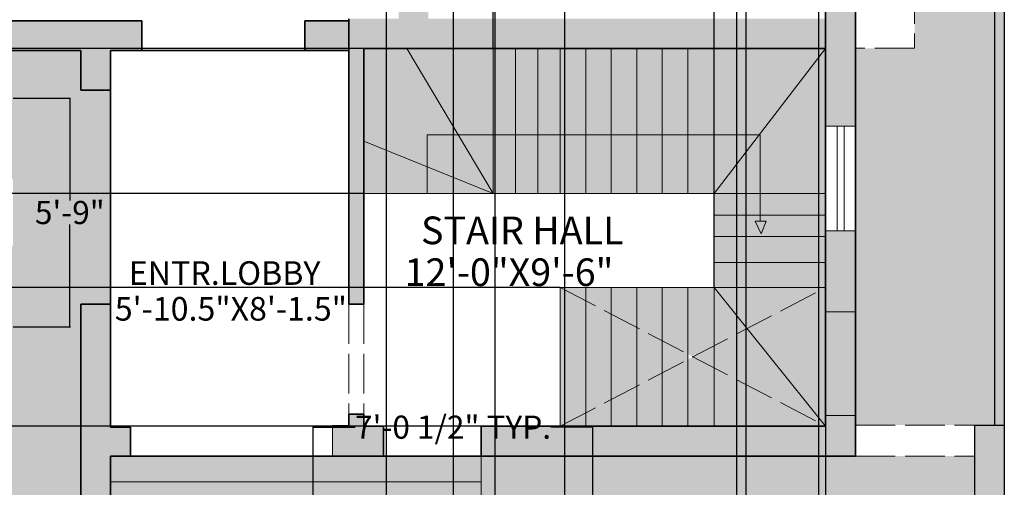
# Model space of a CAD drawing. Units: inches. Extents: x 1884 to 2398, y 474 to 1488.
# Tile 33 of 39: x 2099 to 2397, y 761 to 902. Entities that reach past the tile are written whole.
import ezdxf

# ---------------------------------------------------------------- set-up
doc = ezdxf.new("R2010")
doc.units = ezdxf.units.IN
doc.header["$MEASUREMENT"] = 0
doc.linetypes.add('ACAD_ISO02W100', pattern=[15, 12, -3])
for name, color, linetype, lineweight in [('A-ANNO-DIMS', 2, 'Continuous', 18), ('A-ANNO-SYMB', 7, 'Continuous', 18), ('A-AREA-IDEN', 7, 'Continuous', 18), ('A-FLOR-OVHD', 8, 'ACAD_ISO02W100', 18), ('A-FLOR-PATT', 254, 'Continuous', 13), ('A-FLOR-STRS', 7, 'Continuous', 20), ('A-FLOR-STRS-HIDN', 8, 'ACAD_ISO02W100', 18), ('A-WALL-PATT', 250, 'Continuous', 13), ('C-PROP', 7, 'Continuous', 30), ('walls', 7, 'Continuous', 35), ('windows', 4, 'Continuous', 18)]:
    doc.layers.add(name, color=color, linetype=linetype, lineweight=lineweight)
for name, color, linetype, lineweight, true_color in [('A-FLOR-STRS-PATT', 251, 'Continuous', 13, 0x636466), ('A-GLAZ-PATT', 7, 'Continuous', 13, 0xf5f5f5), ('L-PVMT-PATT', 9, 'Continuous', 13, 0xc7c8ca)]:
    doc.layers.add(name, color=color, linetype=linetype, lineweight=lineweight, true_color=true_color)
doc.styles.get("Standard").update_dxf_attribs({"font": 'arial.ttf'})
doc.dimstyles.get("Standard").update_dxf_attribs({"dimtxt": 7, "dimasz": 0.18, "dimexe": 0.18, "dimexo": 0.0625, "dimgap": 0.09, "dimtad": 0, "dimtih": 1, "dimtoh": 1, "dimzin": 0, "dimdsep": 46, "dimlunit": 3, "dimtxsty": 'Standard', "dimcen": 0.09, "dimadec": 0, "dimazin": 0, "dimtfac": 1, "dimtofl": 0, "dimtmove": 0, "dimatfit": 3, "dimfxl": 1, "dimtolj": 1, "dimtzin": 0, "dimarcsym": 0})

# ---------------------------------------------------------------- blocks, each defined once
blk = doc.blocks.new('*D24')
at = {"layer": 'A-ANNO-DIMS', "color": 0, "lineweight": -2, "transparency": 16777216}
for p, q in [((2187.71, 752.87), (2187.71, 778.86)), ((2187.89, 778.68), (2200.43, 778.68)), ((2272.06, 778.68), (2259.53, 778.68)), ((2272.24, 752.87), (2272.24, 778.86))]:
    blk.add_line(p, q, dxfattribs=at)
at = {"layer": 'A-ANNO-DIMS', "color": 0, "lineweight": 100, "transparency": 16777216}
for points in [[(2187.89, 778.71), (2187.89, 778.65), (2187.71, 778.68)], [(2272.06, 778.71), (2272.06, 778.65), (2272.24, 778.68)]]:
    blk.add_solid(points, dxfattribs=at)
at = {"layer": 'Defpoints', "color": 0, "lineweight": 100, "transparency": 16777216}
for p in [(2272.24, 778.68), (2187.71, 752.81), (2272.24, 752.81)]:
    blk.add_point(p, dxfattribs=at)
at = {"layer": 'A-ANNO-DIMS', "color": 0, "transparency": 16777216, "insert": (2229.98, 778.68), "char_height": 7, "attachment_point": 5}
blk.add_mtext('\\A1;7\'-0 1/2" TYP.', dxfattribs=at)
blk = doc.blocks.new('*D36')
at = {"layer": 'A-ANNO-DIMS', "color": 0, "lineweight": -2, "transparency": 16777216}
for p, q in [((2097.11, 878.02), (2114.37, 878.02)), ((2114.19, 877.84), (2114.19, 847.14)), ((2114.19, 809.11), (2114.19, 839.81)), ((2097.11, 808.93), (2114.37, 808.93))]:
    blk.add_line(p, q, dxfattribs=at)
at = {"layer": 'A-ANNO-DIMS', "color": 0, "lineweight": 100, "transparency": 16777216}
for points in [[(2114.16, 877.84), (2114.22, 877.84), (2114.19, 878.02)], [(2114.16, 809.11), (2114.22, 809.11), (2114.19, 808.93)]]:
    blk.add_solid(points, dxfattribs=at)
at = {"layer": 'Defpoints', "color": 0, "lineweight": 100, "transparency": 16777216}
for p in [(2097.04, 878.02), (2097.04, 808.93), (2114.19, 808.93)]:
    blk.add_point(p, dxfattribs=at)
at = {"layer": 'A-ANNO-DIMS', "color": 0, "transparency": 16777216, "insert": (2114.19, 843.48), "char_height": 7, "attachment_point": 5}
blk.add_mtext('\\A1;5\'-9"', dxfattribs=at)
blk = doc.blocks.new('*D44')
at = {"layer": 'A-ANNO-DIMS', "color": 0, "lineweight": -2, "transparency": 16777216}
for p, q in [((2209.76, 1247.82), (2209.76, 484)), ((2230.03, 1247.82), (2230.03, 484)), ((2209.94, 484.18), (2229.85, 484.18)), ((2230.03, 484.18), (2230.21, 484.18))]:
    blk.add_line(p, q, dxfattribs=at)
at = {"layer": 'A-ANNO-DIMS', "color": 0, "lineweight": 100, "transparency": 16777216}
for points in [[(2209.94, 484.21), (2209.94, 484.15), (2209.76, 484.18)], [(2229.85, 484.21), (2229.85, 484.15), (2230.03, 484.18)]]:
    blk.add_solid(points, dxfattribs=at)
at = {"layer": 'Defpoints', "color": 0, "lineweight": 100, "transparency": 16777216}
for p in [(2209.76, 1247.88), (2230.03, 1247.88), (2230.03, 484.18)]:
    blk.add_point(p, dxfattribs=at)
at = {"layer": 'A-ANNO-DIMS', "color": 0, "transparency": 16777216, "insert": (2247.43, 484.18), "char_height": 7, "attachment_point": 5}
blk.add_mtext('\\A1;1\'-8 1/2"', dxfattribs=at)
blk = doc.blocks.new('*D45')
at = {"layer": 'A-ANNO-DIMS', "color": 0, "lineweight": -2, "transparency": 16777216}
for p, q in [((2242.62, 1322.82), (2242.62, 484)), ((2263.62, 1322.82), (2263.62, 484)), ((2242.8, 484.18), (2244.05, 484.18)), ((2263.44, 484.18), (2262.18, 484.18))]:
    blk.add_line(p, q, dxfattribs=at)
at = {"layer": 'A-ANNO-DIMS', "color": 0, "lineweight": 100, "transparency": 16777216}
for points in [[(2242.8, 484.21), (2242.8, 484.15), (2242.62, 484.18)], [(2263.44, 484.21), (2263.44, 484.15), (2263.62, 484.18)]]:
    blk.add_solid(points, dxfattribs=at)
at = {"layer": 'Defpoints', "color": 0, "lineweight": 100, "transparency": 16777216}
for p in [(2242.62, 1322.88), (2263.62, 1322.88), (2263.62, 484.18)]:
    blk.add_point(p, dxfattribs=at)
at = {"layer": 'A-ANNO-DIMS', "color": 0, "transparency": 16777216, "insert": (2253.12, 484.18), "char_height": 7, "attachment_point": 5}
blk.add_mtext('\\A1;1\'-9"', dxfattribs=at)
blk = doc.blocks.new('*D47')
at = {"layer": 'A-ANNO-DIMS', "color": 0, "lineweight": -2, "transparency": 16777216}
for p, q in [((2315.59, 959.7), (2315.59, 484)), ((2342.53, 959.7), (2342.53, 484)), ((2315.77, 484.18), (2319.61, 484.18)), ((2342.35, 484.18), (2338.51, 484.18))]:
    blk.add_line(p, q, dxfattribs=at)
at = {"layer": 'A-ANNO-DIMS', "color": 0, "lineweight": 100, "transparency": 16777216}
for points in [[(2315.77, 484.21), (2315.77, 484.15), (2315.59, 484.18)], [(2342.35, 484.21), (2342.35, 484.15), (2342.53, 484.18)]]:
    blk.add_solid(points, dxfattribs=at)
at = {"layer": 'Defpoints', "color": 0, "lineweight": 100, "transparency": 16777216}
for p in [(2315.59, 959.77), (2342.53, 959.77), (2342.53, 484.18)]:
    blk.add_point(p, dxfattribs=at)
at = {"layer": 'A-ANNO-DIMS', "color": 0, "transparency": 16777216, "insert": (2329.06, 484.18), "char_height": 7, "attachment_point": 5}
blk.add_mtext('\\A1;2\'-3"', dxfattribs=at)
blk = doc.blocks.new('*D49')
at = {"layer": 'A-ANNO-DIMS', "color": 0, "lineweight": -2, "transparency": 16777216}
for p, q in [((2318.41, 987.72), (2318.41, 484)), ((2340.41, 987.72), (2340.41, 484)), ((2318.59, 484.18), (2340.23, 484.18)), ((2340.41, 484.18), (2340.59, 484.18))]:
    blk.add_line(p, q, dxfattribs=at)
at = {"layer": 'A-ANNO-DIMS', "color": 0, "lineweight": 100, "transparency": 16777216}
for points in [[(2318.59, 484.21), (2318.59, 484.15), (2318.41, 484.18)], [(2340.23, 484.21), (2340.23, 484.15), (2340.41, 484.18)]]:
    blk.add_solid(points, dxfattribs=at)
at = {"layer": 'Defpoints', "color": 0, "lineweight": 100, "transparency": 16777216}
for p in [(2318.41, 987.78), (2340.41, 987.78), (2340.41, 484.18)]:
    blk.add_point(p, dxfattribs=at)
at = {"layer": 'A-ANNO-DIMS', "color": 0, "transparency": 16777216, "insert": (2352.37, 484.18), "char_height": 7, "attachment_point": 5}
blk.add_mtext('\\A1;1\'-10"', dxfattribs=at)
blk = doc.blocks.new('*D51')
at = {"layer": 'A-ANNO-DIMS', "color": 0, "lineweight": -2, "transparency": 16777216}
for p, q in [((2202.97, 892.97), (1902.43, 892.97)), ((1902.61, 892.79), (1902.61, 874.82)), ((1902.61, 849.42), (1902.61, 867.39)), ((2202.97, 849.24), (1902.43, 849.24))]:
    blk.add_line(p, q, dxfattribs=at)
at = {"layer": 'A-ANNO-DIMS', "color": 0, "lineweight": 100, "transparency": 16777216}
for points in [[(1902.58, 892.79), (1902.64, 892.79), (1902.61, 892.97)], [(1902.58, 849.42), (1902.64, 849.42), (1902.61, 849.24)]]:
    blk.add_solid(points, dxfattribs=at)
at = {"layer": 'Defpoints', "color": 0, "lineweight": 100, "transparency": 16777216}
for p in [(1902.61, 892.97), (2203.03, 892.97), (2203.03, 849.24)]:
    blk.add_point(p, dxfattribs=at)
at = {"layer": 'A-ANNO-DIMS', "color": 0, "transparency": 16777216, "insert": (1902.61, 871.1), "char_height": 7, "attachment_point": 5}
blk.add_mtext('\\A1;3\'-7 1/2"', dxfattribs=at)
blk = doc.blocks.new('*D52')
at = {"layer": 'A-ANNO-DIMS', "color": 0, "lineweight": -2, "transparency": 16777216}
for p, q in [((2308.85, 820.89), (2308.85, 1477.76)), ((2309.03, 1477.58), (2342.35, 1477.58)), ((2342.53, 820.89), (2342.53, 1477.76)), ((2342.53, 1477.58), (2342.71, 1477.58))]:
    blk.add_line(p, q, dxfattribs=at)
at = {"layer": 'A-ANNO-DIMS', "color": 0, "lineweight": 100, "transparency": 16777216}
for points in [[(2309.03, 1477.61), (2309.03, 1477.55), (2308.85, 1477.58)], [(2342.35, 1477.61), (2342.35, 1477.55), (2342.53, 1477.58)]]:
    blk.add_solid(points, dxfattribs=at)
at = {"layer": 'Defpoints', "color": 0, "lineweight": 100, "transparency": 16777216}
for p in [(2342.53, 1477.58), (2308.85, 820.83), (2342.53, 820.83)]:
    blk.add_point(p, dxfattribs=at)
at = {"layer": 'A-ANNO-DIMS', "color": 0, "transparency": 16777216, "insert": (2360.32, 1477.58), "char_height": 7, "attachment_point": 5}
blk.add_mtext('\\A1;2\'-9 1/2"', dxfattribs=at)
blk = doc.blocks.new('*D53')
at = {"layer": 'A-ANNO-DIMS', "color": 0, "lineweight": -2, "transparency": 16777216}
for p, q in [((2262.32, 820.83), (1902.43, 820.83)), ((1902.61, 820.65), (1902.61, 803.56)), ((1902.61, 779.15), (1902.61, 796.23)), ((2262.32, 778.97), (1902.43, 778.97))]:
    blk.add_line(p, q, dxfattribs=at)
at = {"layer": 'A-ANNO-DIMS', "color": 0, "lineweight": 100, "transparency": 16777216}
for points in [[(1902.58, 820.65), (1902.64, 820.65), (1902.61, 820.83)], [(1902.58, 779.15), (1902.64, 779.15), (1902.61, 778.97)]]:
    blk.add_solid(points, dxfattribs=at)
at = {"layer": 'Defpoints', "color": 0, "lineweight": 100, "transparency": 16777216}
for p in [(1902.61, 820.83), (2262.38, 820.83), (2262.38, 778.97)]:
    blk.add_point(p, dxfattribs=at)
at = {"layer": 'A-ANNO-DIMS', "color": 0, "transparency": 16777216, "insert": (1902.61, 799.9), "char_height": 7, "attachment_point": 5}
blk.add_mtext('\\A1;3\'-6"', dxfattribs=at)
blk = doc.blocks.new('*D54')
at = {"layer": 'A-ANNO-DIMS', "color": 0, "lineweight": -2, "transparency": 16777216}
for p, q in [((2242.06, 893.03), (2242.06, 1477.76)), ((2242.24, 1477.58), (2266.06, 1477.58)), ((2308.67, 1477.58), (2284.85, 1477.58)), ((2308.85, 893.03), (2308.85, 1477.76))]:
    blk.add_line(p, q, dxfattribs=at)
at = {"layer": 'A-ANNO-DIMS', "color": 0, "lineweight": 100, "transparency": 16777216}
for points in [[(2242.24, 1477.61), (2242.24, 1477.55), (2242.06, 1477.58)], [(2308.67, 1477.61), (2308.67, 1477.55), (2308.85, 1477.58)]]:
    blk.add_solid(points, dxfattribs=at)
at = {"layer": 'Defpoints', "color": 0, "lineweight": 100, "transparency": 16777216}
for p in [(2308.85, 1477.58), (2242.06, 892.97), (2308.85, 892.97)]:
    blk.add_point(p, dxfattribs=at)
at = {"layer": 'A-ANNO-DIMS', "color": 0, "transparency": 16777216, "insert": (2275.45, 1477.58), "char_height": 7, "attachment_point": 5}
blk.add_mtext('\\A1;5\'-7"', dxfattribs=at)

msp = doc.modelspace()

# ---------------------------------------------------------------- hatches: boundary and pattern name
at = {"layer": 'A-ANNO-SYMB'}
h = msp.add_hatch(color=256, dxfattribs=at)
h.dxf.hatch_style = 1
h.paths.add_polyline_path([(2324.539, 840.913), (2323.026, 840.913), (2321.211, 840.913), (2323.026, 837.06)])
at = {"layer": 'A-FLOR-PATT'}
h = msp.add_hatch(color=256, dxfattribs=at)
h.dxf.hatch_style = 1
h.paths.add_polyline_path([(2117.529, 815.801), (2126.529, 815.801), (2126.529, 880.382), (2117.529, 880.382), (2117.529, 892.385), (1961.529, 892.385), (1961.529, 756.915), (1964.529, 756.915), (1964.529, 759.915), (1995.529, 759.915), (1995.529, 753.915), (1972.862, 753.915), (1967.529, 756.915), (1967.529, 654.915), (1972.862, 657.915), (1995.529, 657.915), (1995.529, 651.915), (1964.529, 651.915), (1964.529, 654.915), (1961.529, 654.915), (1961.529, 640.385), (2117.529, 640.385), (2117.529, 646.578), (2126.529, 646.578), (2126.529, 676.183), (2117.529, 676.183)])
h.paths.add_polyline_path([(2012.246, 808.929), (2012.05, 810.185), (2032.542, 810.185), (2032.346, 808.929)], flags=16)
h.paths.add_polyline_path([(2010.381, 820.864), (1994.658, 820.864), (1994.658, 831.561), (1984.608, 833.132), (1984.608, 853.821), (1994.658, 855.391), (1994.658, 866.089), (2010.381, 866.089), (2011.951, 876.139), (2032.64, 876.139), (2034.211, 866.089), (2045.556, 866.089), (2047.127, 876.139), (2067.816, 876.139), (2069.386, 866.089), (2085.109, 866.089), (2085.109, 855.391), (2095.159, 853.821), (2095.159, 833.132), (2085.109, 831.561), (2085.109, 820.864), (2069.386, 820.864), (2067.816, 810.814), (2047.127, 810.814), (2045.556, 820.864), (2034.211, 820.864), (2032.64, 810.814), (2011.951, 810.814)], flags=16)
h.paths.add_polyline_path([(1982.724, 833.426), (1982.724, 853.526), (1983.98, 853.723), (1983.98, 833.23)], flags=16)
h.paths.add_polyline_path([(1994.529, 753.54), (1994.529, 658.29), (1973.529, 658.29), (1973.529, 753.54)], flags=16)
h.paths.add_polyline_path([(2084.486, 843.527), (2084.592, 843.502), (2084.681, 843.487), (2084.813, 843.477), (2084.913, 843.477), (2084.669, 843.482), (2084.336, 843.565), (2084.116, 843.617), (2083.8, 843.686), (2083.105, 843.827), (2082.836, 843.874), (2083.604, 843.729), (2084.206, 843.597)], flags=0)
h.paths.add_polyline_path([(2047.421, 808.929), (2047.225, 810.185), (2067.718, 810.185), (2067.521, 808.929)], flags=16)
h.paths.add_polyline_path([(2066.01, 849.505), (2066.429, 849.687), (2066.798, 849.882), (2067.129, 850.085), (2067.43, 850.293), (2067.711, 850.502), (2068.176, 850.856), (2068.689, 851.205), (2069.305, 851.531), (2070.015, 851.784), (2070.844, 851.944), (2071.081, 851.956), (2070.629, 851.902), (2070.212, 851.822), (2069.827, 851.717), (2069.471, 851.59), (2069.139, 851.443), (2068.828, 851.279), (2068.534, 851.1), (2068.254, 850.909), (2067.983, 850.709), (2067.502, 850.343), (2066.951, 849.962), (2066.224, 849.579)], flags=0)
h.paths.add_polyline_path([(2059.423, 853.221), (2059.827, 853.278), (2060.171, 853.358), (2060.465, 853.463), (2060.714, 853.589), (2060.926, 853.736), (2061.107, 853.902), (2061.258, 854.086), (2061.377, 854.284), (2061.462, 854.495), (2061.514, 854.715), (2061.53, 854.943), (2061.508, 855.176), (2061.449, 855.411), (2061.352, 855.646), (2061.224, 855.882), (2061.07, 856.117), (2060.9, 856.353), (2060.719, 856.588), (2060.406, 856.993), (2060.103, 857.424), (2059.858, 857.888), (2059.691, 858.467), (2059.836, 859.091), (2060.305, 859.532), (2060.844, 859.798), (2061.513, 859.935), (2062.253, 859.905), (2062.483, 859.849), (2062.078, 859.912), (2061.695, 859.928), (2061.336, 859.899), (2061.005, 859.831), (2060.703, 859.729), (2060.437, 859.597), (2060.208, 859.441), (2060.021, 859.265), (2059.879, 859.075), (2059.785, 858.874), (2059.737, 858.664), (2059.73, 858.447), (2059.761, 858.224), (2059.827, 857.996), (2059.923, 857.765), (2060.047, 857.53), (2060.193, 857.295), (2060.359, 857.06), (2060.537, 856.824), (2060.867, 856.399), (2061.171, 855.978), (2061.422, 855.518), (2061.567, 854.943), (2061.41, 854.272), (2060.947, 853.707), (2060.335, 853.397), (2059.649, 853.236)], flags=0)
h.paths.add_polyline_path([(2050.778, 859.745), (2051.07, 859.87), (2051.295, 860.017), (2051.467, 860.183), (2051.594, 860.365), (2051.679, 860.56), (2051.726, 860.763), (2051.739, 860.971), (2051.722, 861.18), (2051.677, 861.387), (2051.609, 861.587), (2051.521, 861.779), (2051.421, 861.962), (2051.312, 862.138), (2051.203, 862.307), (2050.966, 862.68), (2050.793, 863.193), (2051.021, 863.699), (2051.483, 864.018), (2052.09, 864.138), (2052.773, 864.157), (2053.007, 864.142), (2052.603, 864.152), (2052.258, 864.142), (2051.965, 864.113), (2051.716, 864.064), (2051.504, 863.995), (2051.322, 863.907), (2051.17, 863.802), (2051.048, 863.682), (2050.954, 863.55), (2050.891, 863.408), (2050.856, 863.259), (2050.851, 863.105), (2050.876, 862.948), (2050.929, 862.791), (2051.005, 862.633), (2051.098, 862.472), (2051.203, 862.307), (2051.312, 862.138), (2051.556, 861.742), (2051.751, 861.167), (2051.712, 860.535), (2051.398, 860.085), (2050.949, 859.79)], flags=0)
h.paths.add_polyline_path([(2022.768, 719.264), (2050.461, 719.264), (2050.461, 717.226), (2052.426, 717.226), (2052.426, 715.033), (2050.461, 715.033), (2050.461, 703.738), (2022.768, 703.738)], flags=16)
h.paths.add_polyline_path([(2012.246, 878.023), (2032.346, 878.023), (2032.542, 876.767), (2012.05, 876.767)], flags=16)
h.paths.add_polyline_path([(2035.324, 713.103), (2035.342, 713.294), (2035.192, 713.202)], flags=0)
h.paths.add_polyline_path([(2036.484, 711.63), (2036.583, 711.849), (2036.39, 711.898)], flags=0)
h.paths.add_polyline_path([(2036.074, 712.744), (2035.993, 712.481), (2035.724, 712.516), (2035.794, 712.726)], flags=0)
h.paths.add_polyline_path([(2035.846, 710.909), (2035.753, 710.958), (2035.702, 710.88)], flags=0)
h.paths.add_polyline_path([(2037.818, 712.019), (2037.948, 712.06), (2037.987, 712.161), (2037.815, 712.02)], flags=0)
h.paths.add_polyline_path([(2038.451, 709.517), (2038.464, 709.428), (2038.586, 709.442)], flags=0)
h.paths.add_polyline_path([(2037.805, 709.806), (2037.818, 709.807), (2037.804, 709.823)], flags=0)
h.paths.add_polyline_path([(2036.7, 711.245), (2036.698, 711.236), (2036.813, 711.211)], flags=0)
h.paths.add_polyline_path([(2035.928, 708.897), (2035.668, 708.871), (2035.706, 708.667)], flags=0)
h.paths.add_polyline_path([(2036.414, 710.976), (2035.932, 709.859), (2036.792, 710.484), (2036.5, 710.934)], flags=0)
h.paths.add_polyline_path([(2038.298, 712.115), (2038.499, 712.058), (2038.612, 712.269), (2038.39, 712.332)], flags=0)
h.paths.add_polyline_path([(2047.421, 878.023), (2067.521, 878.023), (2067.718, 876.767), (2047.225, 876.767)], flags=16)
h.paths.add_polyline_path([(2049.647, 705.093, -1), (2048.845, 705.093, -1)], flags=0)
h.paths.add_polyline_path([(2095.787, 853.723), (2097.043, 853.526), (2097.043, 833.426), (2095.787, 833.23)], flags=16)
h.paths.add_polyline_path([(2110.739, 745.339), (2111.75, 745.339, -0.0640419), (2113.267, 742.92), (2113.267, 732.192), (2113.526, 732.192, -0.4142136), (2114.278, 731.439), (2114.278, 716.764, -0.4142136), (2113.526, 716.011), (2113.267, 716.011), (2113.267, 705.284, -0.0640419), (2111.75, 702.864), (2110.739, 702.864), (2110.739, 716.011), (2109.469, 716.011, -0.4142136), (2108.716, 716.764), (2108.716, 731.439, -0.4142136), (2109.469, 732.192), (2110.739, 732.192)], flags=16)
h.paths.add_polyline_path([(1998.045, 668.909), (2002.449, 668.909), (2002.449, 652.273), (2002.724, 652.763), (2002.724, 668.175), (2019.972, 668.175), (2019.972, 652.763), (2020.247, 652.273), (2020.247, 668.909), (2024.651, 668.909), (2029.055, 668.909), (2029.055, 652.273), (2029.33, 652.763), (2029.33, 668.175), (2046.578, 668.175), (2046.578, 652.763), (2046.853, 652.273), (2046.853, 668.909), (2051.257, 668.909), (2051.257, 646.157), (2049.055, 646.157), (2049.055, 643.955), (2026.853, 643.955), (2026.853, 646.157), (2024.651, 646.157), (2022.449, 646.157), (2022.449, 643.955), (2000.247, 643.955), (2000.247, 646.157), (1998.045, 646.157)], flags=16)
h.paths.add_polyline_path([(2342.529, 1247.885), (2265.892, 1247.885), (2230.029, 1247.885), (2209.755, 1247.885), (2168.6, 1247.885), (2168.6, 1104.929), (2158.029, 1104.929), (2158.029, 1079.411), (2168.6, 1079.411), (2168.6, 1062.466), (2342.529, 1062.466), (2342.529, 1093.809)])
h.paths.add_polyline_path([(2215.03, 1153.876), (2215.03, 1164.739), (2187.559, 1164.739), (2187.442, 1152.641), (2173.568, 1152.641), (2173.684, 1164.739), (2173.684, 1218.739), (2173.801, 1230.837), (2187.675, 1230.837), (2187.559, 1218.739), (2215.03, 1218.739), (2215.03, 1225.879), (2245.053, 1225.879), (2245.053, 1153.876)], flags=16)
h.paths.add_polyline_path([(2192.147, 1164.797), (2184.963, 1174.54), (2184.915, 1174.54), (2176.755, 1174.54), (2176.755, 1190.363), (2184.915, 1190.363), (2184.915, 1196.819), (2176.755, 1196.819), (2176.755, 1212.641), (2184.915, 1212.641), (2184.915, 1174.606), (2184.963, 1174.54), (2192.147, 1174.54)], flags=0)
h.paths.add_polyline_path([(2184.971, 1158.364, -1), (2176.039, 1158.364, -1)], flags=0)
h.paths.add_polyline_path([(2335.555, 1161.985), (2335.555, 1175.132), (2334.285, 1175.132, -0.4142136), (2333.533, 1175.885), (2333.533, 1190.56, -0.4142136), (2334.285, 1191.313), (2335.555, 1191.313), (2335.555, 1204.46), (2336.567, 1204.46, -0.0640419), (2338.083, 1202.04), (2338.083, 1191.313), (2338.342, 1191.313, -0.4142136), (2339.095, 1190.56), (2339.095, 1175.885, -0.4142136), (2338.342, 1175.132), (2338.083, 1175.132), (2338.083, 1164.405, -0.0640419), (2336.567, 1161.985)], flags=16)
h.paths.add_polyline_path([(2176.155, 1224.462, -1), (2185.087, 1224.462, -1)], flags=0)
h.paths.add_polyline_path([(2158.029, 1276.197), (2158.029, 1322.885), (2148.233, 1322.885), (2092.029, 1322.885), (1961.529, 1322.885), (1961.529, 1166.885), (2116.005, 1166.885), (2116.005, 1157.885), (2152.638, 1157.885), (2152.638, 1166.885), (2158.029, 1166.885)])
h.paths.add_polyline_path([(2006.352, 1204.245), (2006.352, 1215.108), (1978.881, 1215.108), (1978.764, 1203.01), (1964.89, 1203.01), (1965.006, 1215.108), (1965.006, 1269.108), (1965.123, 1281.207), (1978.997, 1281.207), (1978.881, 1269.108), (2006.352, 1269.108), (2006.352, 1276.248), (2036.375, 1276.248), (2036.375, 1204.245)], flags=16)
h.paths.add_polyline_path([(1983.469, 1215.166), (1976.285, 1224.909), (1976.237, 1224.909), (1968.077, 1224.909), (1968.077, 1240.732), (1976.237, 1240.732), (1976.237, 1247.188), (1968.077, 1247.188), (1968.077, 1263.011), (1976.237, 1263.011), (1976.237, 1224.975), (1976.285, 1224.909), (1983.469, 1224.909)], flags=0)
h.paths.add_polyline_path([(1976.293, 1208.733, -1), (1967.361, 1208.733, -1)], flags=0)
h.paths.add_polyline_path([(1967.477, 1274.832, -1), (1976.41, 1274.832, -1)], flags=0)
h.paths.add_polyline_path([(2152.587, 1223.485), (2152.587, 1236.632), (2151.317, 1236.632, -0.4142136), (2150.564, 1237.385), (2150.564, 1252.06, -0.4142136), (2151.317, 1252.813), (2152.587, 1252.813), (2152.587, 1265.959), (2153.598, 1265.959, -0.0640419), (2155.115, 1263.54), (2155.115, 1252.813), (2155.374, 1252.813, -0.4142136), (2156.126, 1252.06), (2156.126, 1237.385, -0.4142136), (2155.374, 1236.632), (2155.115, 1236.632), (2155.115, 1225.904, -0.0640419), (2153.598, 1223.485)], flags=16)
h.paths.add_polyline_path([(2250.676, 1161.101), (2322.077, 1161.101), (2322.077, 1173.886), (2250.676, 1173.886)], flags=24)
h.paths.add_polyline_path([(2255.61, 1173.712), (2320.136, 1173.712), (2320.136, 1186.659), (2255.61, 1186.659)], flags=24)
h.paths.add_polyline_path([(2053.687, 1230.837), (2125.089, 1230.837), (2125.089, 1243.622), (2053.687, 1243.622)], flags=24)
h.paths.add_polyline_path([(2058.622, 1243.448), (2123.147, 1243.448), (2123.147, 1256.395), (2058.622, 1256.395)], flags=24)
at = {"layer": 'A-FLOR-STRS-PATT'}
h = msp.add_hatch(color=256, dxfattribs=at)
h.dxf.hatch_style = 1
h.paths.add_polyline_path([(2215.996, 892.966), (2203.029, 892.966), (2203.029, 865.024), (2222.194, 857.274), (2222.194, 866.959), (2231.498, 866.959)])
h.paths.add_polyline_path([(2242.059, 892.966), (2215.996, 892.966), (2231.498, 866.959), (2242.059, 866.959)])
h.paths.add_polyline_path([(2231.498, 866.959), (2222.194, 866.959), (2222.194, 857.274), (2242.059, 849.241)])
h.paths.add_polyline_path([(2242.059, 866.959), (2231.498, 866.959), (2242.059, 849.241)], flags=17)
h.paths.add_polyline_path([(2222.194, 857.274), (2203.029, 865.024), (2203.029, 849.241), (2222.194, 849.241)])
h.paths.add_polyline_path([(2222.194, 857.274), (2222.194, 849.241), (2242.059, 849.241)], flags=17)
h.paths.add_polyline_path([(2248.833, 866.959), (2242.059, 866.959), (2242.059, 849.241), (2248.833, 849.241)])
h.paths.add_polyline_path([(2248.833, 892.966), (2242.059, 892.966), (2242.059, 866.959), (2248.833, 866.959)])
h.paths.add_polyline_path([(2255.607, 866.959), (2248.833, 866.959), (2248.833, 849.241), (2255.607, 849.241)])
h.paths.add_polyline_path([(2255.607, 892.966), (2248.833, 892.966), (2248.833, 866.959), (2255.607, 866.959)])
h.paths.add_polyline_path([(2262.382, 866.959), (2255.607, 866.959), (2255.607, 849.241), (2262.382, 849.241)])
h.paths.add_polyline_path([(2262.382, 892.966), (2255.607, 892.966), (2255.607, 866.959), (2262.382, 866.959)])
h.paths.add_polyline_path([(2270.083, 866.959), (2262.382, 866.959), (2262.382, 849.241), (2270.083, 849.241)])
h.paths.add_polyline_path([(2270.083, 892.966), (2262.382, 892.966), (2262.382, 866.959), (2270.083, 866.959)])
h.paths.add_polyline_path([(2277.785, 866.959), (2270.083, 866.959), (2270.083, 849.241), (2277.785, 849.241)])
h.paths.add_polyline_path([(2277.785, 892.966), (2270.083, 892.966), (2270.083, 866.959), (2277.785, 866.959)])
h.paths.add_polyline_path([(2285.487, 866.959), (2277.785, 866.959), (2277.785, 849.241), (2285.487, 849.241)])
h.paths.add_polyline_path([(2285.487, 892.966), (2277.785, 892.966), (2277.785, 866.959), (2285.487, 866.959)])
h.paths.add_polyline_path([(2293.189, 866.959), (2285.487, 866.959), (2285.487, 849.241), (2293.189, 849.241)])
h.paths.add_polyline_path([(2293.189, 892.966), (2285.487, 892.966), (2285.487, 866.959), (2293.189, 866.959)])
h.paths.add_polyline_path([(2300.89, 866.959), (2293.189, 866.959), (2293.189, 849.241), (2300.89, 849.241)])
h.paths.add_polyline_path([(2300.89, 892.966), (2293.189, 892.966), (2293.189, 866.959), (2300.89, 866.959)])
h.paths.add_polyline_path([(2308.846, 866.959), (2300.89, 866.959), (2300.89, 849.241), (2308.846, 849.241)])
h.paths.add_polyline_path([(2308.846, 892.966), (2300.89, 892.966), (2300.89, 866.959), (2308.846, 866.959)])
h.paths.add_polyline_path([(2322.733, 866.959), (2322.495, 866.959), (2308.846, 849.241), (2322.733, 849.241)])
h.paths.add_polyline_path([(2342.529, 892.966), (2308.846, 892.966), (2308.846, 866.959), (2322.495, 866.959)])
h.paths.add_polyline_path([(2322.495, 866.959), (2308.846, 866.959), (2308.846, 849.241)], flags=17)
h.paths.add_polyline_path([(2342.529, 869.555), (2342.529, 892.966), (2322.495, 866.959), (2322.733, 866.959), (2322.733, 849.241), (2342.529, 849.241)])
h.paths.add_polyline_path([(2342.529, 849.241), (2322.733, 849.241), (2322.733, 842.717), (2342.529, 842.717)])
h.paths.add_polyline_path([(2321.211, 840.913), (2322.733, 840.913), (2322.733, 842.717), (2308.846, 842.717), (2308.846, 840.204), (2308.846, 836.194), (2342.529, 836.194), (2342.529, 842.717), (2322.733, 842.717), (2322.733, 840.913), (2323.026, 840.913), (2324.539, 840.913), (2323.026, 837.06)])
h.paths.add_polyline_path([(2322.733, 849.241), (2308.846, 849.241), (2308.846, 842.717), (2322.733, 842.717)])
h.paths.add_polyline_path([(2342.529, 836.194), (2308.846, 836.194), (2308.846, 828.397), (2342.529, 828.397)])
h.paths.add_polyline_path([(2342.529, 828.397), (2308.846, 828.397), (2308.846, 820.826), (2342.529, 820.826)])
h.paths.add_polyline_path([(2342.529, 820.826), (2318.813, 808.439), (2342.529, 778.966)])
h.paths.add_polyline_path([(2342.529, 820.826), (2308.846, 820.826), (2318.813, 808.439)])
h.paths.add_polyline_path([(2318.813, 808.439), (2308.846, 803.234), (2308.846, 796.559), (2342.529, 778.966)])
h.paths.add_polyline_path([(2308.846, 820.826), (2308.846, 811.789), (2308.846, 803.234), (2318.813, 808.439)])
h.paths.add_polyline_path([(2308.846, 811.789), (2308.846, 820.826), (2300.89, 820.826), (2300.89, 800.714), (2302.455, 799.896), (2308.846, 803.234)])
h.paths.add_polyline_path([(2308.846, 796.559), (2308.846, 778.966), (2342.529, 778.966)], flags=17)
h.paths.add_polyline_path([(2308.846, 796.559), (2302.455, 799.896), (2300.89, 799.079), (2300.89, 778.966), (2308.846, 778.966)])
h.paths.add_polyline_path([(2308.846, 803.234), (2302.455, 799.896), (2308.846, 796.559)])
h.paths.add_polyline_path([(2300.89, 799.079), (2293.189, 795.056), (2293.189, 778.966), (2300.89, 778.966)])
h.paths.add_polyline_path([(2300.89, 800.714), (2293.189, 804.736), (2293.189, 795.056), (2300.89, 799.079)])
h.paths.add_polyline_path([(2300.89, 820.826), (2293.189, 820.826), (2293.189, 804.736), (2300.89, 800.714)])
h.paths.add_polyline_path([(2293.189, 820.826), (2285.487, 820.826), (2285.487, 808.759), (2293.189, 804.736)])
h.paths.add_polyline_path([(2293.189, 804.736), (2285.487, 808.759), (2285.487, 791.034), (2293.189, 795.056)])
h.paths.add_polyline_path([(2293.189, 795.056), (2285.487, 791.034), (2285.487, 778.966), (2293.189, 778.966)])
h.paths.add_polyline_path([(2285.487, 791.034), (2277.785, 787.011), (2277.785, 778.966), (2285.487, 778.966)])
h.paths.add_polyline_path([(2285.487, 808.759), (2277.785, 812.781), (2277.785, 787.011), (2285.487, 791.034)])
h.paths.add_polyline_path([(2285.487, 820.826), (2277.785, 820.826), (2277.785, 812.781), (2285.487, 808.759)])
h.paths.add_polyline_path([(2277.785, 820.826), (2270.083, 820.826), (2270.083, 816.804), (2277.785, 812.781)])
h.paths.add_polyline_path([(2277.785, 812.781), (2270.083, 816.804), (2270.083, 782.989), (2277.785, 787.011)])
h.paths.add_polyline_path([(2277.785, 787.011), (2270.083, 782.989), (2270.083, 778.966), (2277.785, 778.966)])
h.paths.add_polyline_path([(2270.083, 816.804), (2262.382, 820.826), (2262.382, 778.966), (2270.083, 782.989)])
h.paths.add_polyline_path([(2270.083, 782.989), (2262.382, 778.966), (2270.083, 778.966)], flags=17)
h.paths.add_polyline_path([(2270.083, 820.826), (2262.382, 820.826), (2270.083, 816.804)], flags=0)
h = msp.add_hatch(color=256, dxfattribs=at)
h.dxf.hatch_style = 1
h.paths.add_polyline_path([(2270.083, 820.826), (2262.382, 820.826), (2270.083, 816.804)])
h = msp.add_hatch(color=256, dxfattribs=at)
h.dxf.hatch_style = 1
h.paths.add_polyline_path([(2238.447, 769.966), (2198.529, 769.966), (2193.526, 769.966), (2132.515, 769.966), (2126.529, 769.966), (2126.529, 762.15), (2238.447, 762.15)])
h.paths.add_polyline_path([(2238.447, 762.15), (2126.529, 762.15), (2126.529, 754.445), (2238.447, 754.445)])
at = {"layer": 'A-GLAZ-PATT'}
h = msp.add_hatch(color=256, dxfattribs=at)
h.dxf.hatch_style = 1
h.paths.add_polyline_path([(2351.529, 813.478), (2342.529, 813.478), (2342.529, 782.175), (2351.529, 782.175)])
at = {"layer": 'A-WALL-PATT'}
h = msp.add_hatch(color=256, dxfattribs=at)
h.dxf.hatch_style = 1
h.paths.add_polyline_path([(2396.529, 1406.885), (2393.529, 1406.885), (2393.529, 779.322), (2396.529, 779.322)])
h = msp.add_hatch(color=256, dxfattribs=at)
h.dxf.hatch_style = 1
h.paths.add_polyline_path([(2351.529, 837.963), (2342.529, 837.963), (2342.529, 813.478), (2351.529, 813.478)])
h.paths.add_polyline_path([(2351.529, 782.175), (2342.529, 782.175), (2342.529, 778.966), (2238.447, 778.966), (2238.447, 769.966), (2351.529, 769.966)])
h.paths.add_polyline_path([(2351.529, 914.773), (2342.529, 914.773), (2342.529, 901.966), (2222.529, 901.966), (2222.529, 908.236), (2213.529, 908.236), (2213.529, 901.966), (2198.529, 901.966), (2198.529, 892.966), (2198.529, 815.857), (2203.029, 815.857), (2203.029, 892.966), (2342.529, 892.966), (2342.529, 869.555), (2346.047, 869.555), (2351.529, 869.555), (2351.529, 880.385)])
h.paths.add_polyline_path([(2208.948, 778.966), (2203.029, 778.966), (2203.029, 782.647), (2198.529, 782.647), (2198.529, 779.109), (2193.526, 779.109), (2193.526, 769.966), (2198.529, 769.966), (2208.948, 769.966)])
h.paths.add_polyline_path([(2126.529, 815.801), (2117.529, 815.801), (2117.529, 676.183), (2126.529, 676.183), (2126.529, 769.966), (2132.515, 769.966), (2132.515, 778.664), (2126.529, 778.664)])
h.paths.add_polyline_path([(2135.996, 901.385), (2009.529, 901.385), (2009.529, 929.544), (2000.529, 929.544), (2000.529, 892.385), (2117.529, 892.385), (2117.529, 880.382), (2126.529, 880.382), (2126.529, 892.385), (2135.996, 892.385)])
h.paths.add_polyline_path([(2198.529, 901.385), (2185.2, 901.385), (2185.2, 892.385), (2198.529, 892.385), (2198.529, 892.966)])
h.paths.add_polyline_path([(1961.529, 892.385), (1965.143, 892.385), (1965.143, 901.385), (1952.529, 901.385), (1952.529, 604.13), (1961.529, 604.13), (1961.529, 631.385), (1988.002, 631.385), (1988.002, 640.385), (1961.529, 640.385)])
h.paths.add_polyline_path([(1955.529, 604.13), (1952.529, 604.13), (1952.529, 530.885), (2126.529, 530.885), (2126.529, 533.885), (1955.529, 533.885)])
h.paths.add_polyline_path([(2396.529, 604.13), (2393.529, 604.13), (2393.529, 533.885), (2126.529, 533.885), (2126.529, 530.885), (2396.529, 530.885)])
h.paths.add_polyline_path([(2396.529, 779.322), (2387.529, 779.322), (2387.529, 604.13), (2396.529, 604.13)])
at = {"layer": 'L-PVMT-PATT'}
h = msp.add_hatch(color=256, dxfattribs=at)
h.dxf.hatch_style = 1
h.paths.add_polyline_path([(2393.529, 1403.885), (2170.029, 1403.885), (2170.029, 1343.885), (2265.892, 1343.885), (2351.529, 1343.885), (2351.529, 1276.197), (2351.529, 1062.466), (2369.436, 1062.466), (2369.436, 893.06), (2351.529, 893.06), (2351.529, 880.385), (2351.529, 779.322), (2387.529, 779.322), (2393.529, 779.322)])
h = msp.add_hatch(color=256, dxfattribs=at)
h.dxf.hatch_style = 1
h.paths.add_polyline_path([(2387.529, 769.966), (2351.529, 769.966), (2238.447, 769.966), (2238.447, 762.15), (2238.447, 754.445), (2126.529, 754.445), (2126.529, 676.183), (2134.868, 676.183), (2142.673, 676.183), (2142.673, 646.578), (2134.868, 646.578), (2126.529, 646.578), (2126.529, 640.17), (2387.529, 640.17)])
h.paths.add_polyline_path([(2387.529, 631.385), (2303.086, 631.385), (2303.086, 615.671), (2387.529, 615.671)])
h.paths.add_polyline_path([(2387.529, 640.17), (2126.529, 640.17), (2126.529, 631.385), (2387.529, 631.385)])
h.paths.add_polyline_path([(2393.529, 604.13), (2387.529, 604.13), (2387.529, 615.671), (2303.086, 615.671), (2303.086, 607.943), (2249.649, 607.943), (2126.529, 607.943), (2126.529, 533.885), (2393.529, 533.885)])
h.paths.add_polyline_path([(2257.825, 611.008), (2257.83, 611.337), (2257.915, 616.493), (2258.021, 621.805), (2258.146, 627.274), (2258.252, 631.385), (2126.529, 631.385), (2126.529, 611.008)])
h.paths.add_polyline_path([(2258.892, 611.285), (2258.888, 611.008), (2300.247, 611.008), (2300.247, 631.385), (2259.314, 631.385), (2259.206, 627.173), (2259.081, 621.72), (2258.976, 616.424)])

# ---------------------------------------------------------------- linework, layer by layer
at = {"layer": 'A-ANNO-SYMB'}
for p, q in [((2222.194, 849.241), (2222.194, 866.959)), ((2222.194, 866.959), (2322.733, 866.959)), ((2322.733, 866.959), (2322.733, 840.913)), ((2323.026, 837.06), (2321.211, 840.913)), ((2321.211, 840.913), (2323.026, 840.913)), ((2323.026, 840.913), (2324.539, 840.913)), ((2324.539, 840.913), (2323.026, 837.06))]:
    msp.add_line(p, q, dxfattribs=at)
at = {"layer": 'A-FLOR-OVHD'}
for p, q in [((2369.436, 1062.466), (2369.436, 893.06)), ((2369.436, 893.06), (2351.529, 893.06)), ((2198.529, 815.857), (2198.529, 782.647)), ((2203.029, 815.857), (2203.029, 782.647)), ((2193.526, 779.109), (2193.526, 769.966)), ((2351.529, 779.322), (2387.529, 779.322)), ((2351.529, 769.966), (2387.529, 769.966))]:
    msp.add_line(p, q, dxfattribs=at)
at = {"layer": 'A-FLOR-STRS'}
for p, q in [((2242.059, 849.241), (2215.996, 892.966)), ((2242.059, 892.966), (2242.059, 849.241)), ((2248.833, 892.966), (2248.833, 849.241)), ((2255.607, 892.966), (2255.607, 849.241)), ((2262.382, 892.966), (2262.382, 849.241)), ((2270.083, 892.966), (2270.083, 849.241)), ((2277.785, 892.966), (2277.785, 849.241)), ((2285.487, 892.966), (2285.487, 849.241)), ((2293.189, 892.966), (2293.189, 849.241)), ((2300.89, 892.966), (2300.89, 849.241)), ((2308.846, 892.966), (2308.846, 836.194)), ((2308.846, 849.241), (2342.529, 892.966)), ((2242.059, 849.241), (2203.029, 865.024)), ((2203.029, 849.241), (2308.846, 849.241)), ((2308.846, 849.241), (2342.529, 849.241)), ((2308.846, 842.717), (2342.529, 842.717)), ((2308.846, 842.717), (2308.846, 820.826)), ((2308.846, 840.204), (2308.846, 811.789)), ((2308.846, 836.194), (2342.529, 836.194)), ((2308.846, 828.397), (2342.529, 828.397)), ((2308.846, 820.826), (2262.382, 820.826)), ((2262.382, 820.826), (2262.382, 778.966)), ((2270.083, 820.826), (2270.083, 778.966)), ((2277.785, 820.826), (2277.785, 778.966)), ((2285.487, 820.826), (2285.487, 778.966)), ((2293.189, 820.826), (2293.189, 778.966)), ((2300.89, 820.826), (2300.89, 778.966)), ((2308.846, 820.826), (2308.846, 778.966)), ((2308.846, 820.826), (2342.529, 820.826)), ((2308.846, 820.826), (2342.529, 778.966)), ((2238.447, 762.15), (2238.447, 769.966)), ((2126.529, 762.15), (2238.447, 762.15)), ((2238.447, 754.445), (2238.447, 762.15))]:
    msp.add_line(p, q, dxfattribs=at)
at = {"layer": 'A-FLOR-STRS-HIDN'}
for p, q in [((2262.382, 820.826), (2342.529, 778.966)), ((2262.382, 778.966), (2342.529, 820.826))]:
    msp.add_line(p, q, dxfattribs=at)
at = {"layer": 'C-PROP'}
for p, q in [((2396.529, 1406.885), (2396.529, 530.885)), ((2393.529, 1403.885), (2393.529, 779.322)), ((2387.529, 779.322), (2387.529, 604.13)), ((2387.529, 779.322), (2396.529, 779.322))]:
    msp.add_line(p, q, dxfattribs=at)
at = {"layer": 'walls'}
for p, q in [((2351.529, 922.094), (2351.529, 880.385)), ((2009.529, 901.385), (2135.996, 901.385)), ((2135.996, 901.385), (2135.996, 892.385)), ((2185.2, 901.385), (2185.2, 892.385)), ((2185.2, 901.385), (2198.529, 901.385)), ((2198.529, 892.966), (2198.529, 901.966)), ((2198.529, 892.966), (2198.529, 815.857)), ((2342.529, 892.966), (2203.029, 892.966)), ((2203.029, 892.966), (2203.029, 815.857)), ((2342.529, 892.966), (2342.529, 778.966)), ((1961.529, 892.385), (2117.529, 892.385)), ((2117.529, 880.382), (2117.529, 892.385)), ((2126.529, 892.385), (2198.529, 892.385)), ((2126.529, 778.664), (2126.529, 892.385)), ((2117.529, 880.382), (2126.529, 880.382)), ((2351.529, 880.385), (2351.529, 769.966)), ((2117.529, 815.801), (2126.529, 815.801)), ((2117.529, 676.183), (2117.529, 815.801)), ((2198.529, 815.857), (2203.029, 815.857)), ((2198.529, 782.647), (2203.029, 782.647)), ((2198.529, 782.647), (2198.529, 779.109)), ((2203.029, 782.647), (2203.029, 778.966)), ((2126.529, 778.664), (2132.515, 778.664)), ((2132.515, 778.664), (2132.515, 769.966)), ((2198.529, 779.109), (2193.526, 779.109)), ((2208.948, 778.966), (2203.029, 778.966)), ((2208.948, 778.966), (2208.948, 769.966)), ((2342.529, 778.966), (2238.447, 778.966)), ((2238.447, 769.966), (2238.447, 778.966)), ((2126.529, 530.885), (2126.529, 769.966)), ((2132.515, 769.966), (2126.529, 769.966)), ((2132.515, 769.966), (2193.526, 769.966)), ((2193.526, 769.966), (2198.529, 769.966)), ((2351.529, 769.966), (2198.529, 769.966))]:
    msp.add_line(p, q, dxfattribs=at)
at = {"layer": 'windows'}
for p, q in [((2342.529, 869.555), (2351.529, 869.555)), ((2342.529, 837.963), (2342.529, 869.555)), ((2342.529, 869.555), (2346.047, 869.555)), ((2346.047, 869.555), (2346.047, 837.963)), ((2348.148, 837.963), (2348.148, 869.555)), ((2351.529, 869.555), (2351.529, 837.963)), ((2351.529, 837.963), (2342.529, 837.963)), ((2346.047, 837.963), (2348.148, 837.963)), ((2342.529, 813.478), (2351.529, 813.478)), ((2342.529, 782.175), (2342.529, 813.478)), ((2351.529, 813.478), (2351.529, 782.175)), ((2351.529, 782.175), (2342.529, 782.175))]:
    msp.add_line(p, q, dxfattribs=at)

# ---------------------------------------------------------------- texts
at = {"layer": 'A-AREA-IDEN'}
for s, height, p in [('STAIR HALL', 8.3413, (2220.297, 833.916)), ('12\'-0"X9\'-6"', 8.34125, (2215.335, 821.284)), ('ENTR.LOBBY', 7.1289, (2132.021, 821.641)), ('5\'-10.5"X8\'-1.5"', 7.12892, (2127.781, 810.844))]:
    msp.add_text(s, height=height, dxfattribs=at).set_placement(p)

# ---------------------------------------------------------------- dimensions: what is measured, and where the dimension line sits
at = {"layer": 'A-ANNO-DIMS'}
for base, p1, p2, picture, middle in [((2342.529, 1477.585), (2308.846, 820.826), (2342.529, 820.826), '*D52', (2360.318, 1477.585)), ((2308.846, 1477.585), (2242.059, 892.966), (2308.846, 892.966), '*D54', (2275.452, 1477.585)), ((2263.617, 484.185), (2242.617, 1322.885), (2263.617, 1322.885), '*D45', (2253.117, 484.185)), ((2230.029, 484.185), (2209.755, 1247.885), (2230.029, 1247.885), '*D44', (2247.429, 484.185)), ((2340.409, 484.185), (2318.409, 987.778), (2340.409, 987.778), '*D49', (2352.373, 484.185)), ((2342.529, 484.185), (2315.591, 959.766), (2342.529, 959.766), '*D47', (2329.06, 484.185))]:
    dim = msp.add_linear_dim(base=base, p1=p1, p2=p2, dimstyle='Standard', override={"dimdec": 1, "dimlfac": 1, "dimrnd": 0, "dimzin": 1, "dimdsep": 46, "dimlunit": 4, "dimfrac": 2}, dxfattribs=at)
    dim.commit()
    dim.dimension.update_dxf_attribs({"geometry": picture, "text_midpoint": middle})
for base, p1, p2, angle, picture, middle in [((1902.612, 892.966), (2203.029, 849.241), (2203.029, 892.966), 90, '*D51', (1902.612, 871.103)), ((2114.191, 808.929), (2097.043, 878.023), (2097.043, 808.929), 270, '*D36', (2114.191, 843.476)), ((1902.612, 820.826), (2262.382, 778.966), (2262.382, 820.826), 90, '*D53', (1902.612, 799.896))]:
    dim = msp.add_linear_dim(base=base, p1=p1, p2=p2, angle=angle, dimstyle='Standard', override={"dimdec": 1, "dimlfac": 1, "dimrnd": 0, "dimzin": 1, "dimdsep": 46, "dimlunit": 4, "dimfrac": 2}, dxfattribs=at)
    dim.commit()
    dim.dimension.update_dxf_attribs({"geometry": picture, "text_midpoint": middle})
dim = msp.add_linear_dim(base=(2272.242, 778.681), p1=(2187.713, 752.812), p2=(2272.242, 752.812), text='<> TYP.', dimstyle='Standard', override={"dimdec": 1, "dimlfac": 1, "dimrnd": 0, "dimzin": 1, "dimdsep": 46, "dimlunit": 4, "dimfrac": 2}, dxfattribs=at)
dim.commit()
dim.dimension.update_dxf_attribs({"geometry": '*D24', "text_midpoint": (2229.977, 778.681)})

doc.saveas('drawing.dxf')
